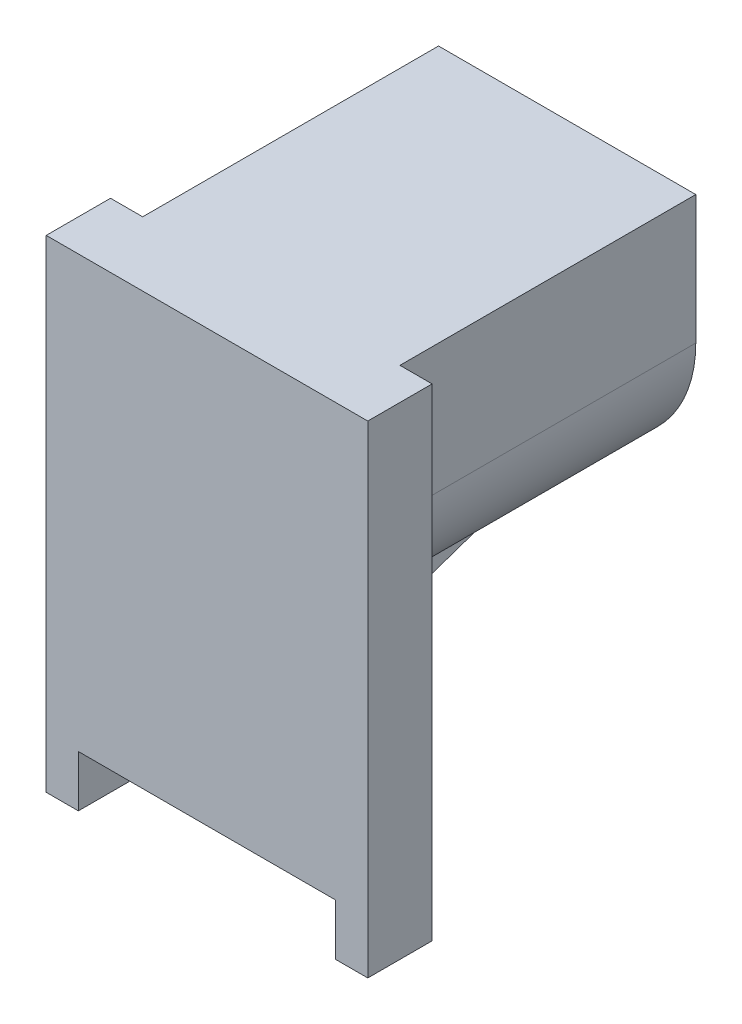
ISO-10303-21;
HEADER;
FILE_DESCRIPTION(('STEP AP214'),'2;1');
FILE_NAME('part.step','',(''),(''),'','','');
FILE_SCHEMA(('AUTOMOTIVE_DESIGN { 1 0 10303 214 1 1 1 1 }'));
ENDSEC;
DATA;
#1=APPLICATION_CONTEXT('core data for automotive mechanical design processes');
#2=APPLICATION_PROTOCOL_DEFINITION('international standard','automotive_design',2000,#1);
#3=PRODUCT_CONTEXT('',#1,'mechanical');
#4=PRODUCT('Part','Part','',(#3));
#5=PRODUCT_RELATED_PRODUCT_CATEGORY('part','',(#4));
#6=PRODUCT_DEFINITION_FORMATION('','',#4);
#7=PRODUCT_DEFINITION_CONTEXT('part definition',#1,'design');
#8=PRODUCT_DEFINITION('design','',#6,#7);
#9=PRODUCT_DEFINITION_SHAPE('','',#8);
#10=(LENGTH_UNIT() NAMED_UNIT(*) SI_UNIT(.MILLI.,.METRE.));
#11=(NAMED_UNIT(*) PLANE_ANGLE_UNIT() SI_UNIT($,.RADIAN.));
#12=(NAMED_UNIT(*) SI_UNIT($,.STERADIAN.) SOLID_ANGLE_UNIT());
#13=UNCERTAINTY_MEASURE_WITH_UNIT(LENGTH_MEASURE(1.E-05),#10,'distance_accuracy_value','');
#14=(GEOMETRIC_REPRESENTATION_CONTEXT(3) GLOBAL_UNCERTAINTY_ASSIGNED_CONTEXT((#13)) GLOBAL_UNIT_ASSIGNED_CONTEXT((#10,
#11,#12)) REPRESENTATION_CONTEXT('',''));
#15=CARTESIAN_POINT('',(0.,0.,0.));
#16=DIRECTION('',(0.,0.,1.));
#17=DIRECTION('',(1.,0.,0.));
#18=AXIS2_PLACEMENT_3D('',#15,#16,#17);
#19=CARTESIAN_POINT('',(100.,-79.3050321097279,0.));
#20=DIRECTION('',(0.,0.999971469772017,-0.00755378328999664));
#21=DIRECTION('',(0.,0.00755378328999664,0.999971469772017));
#22=AXIS2_PLACEMENT_3D('',#19,#20,#21);
#23=PLANE('',#22);
#24=DIRECTION('',(-1.,0.,0.));
#25=VECTOR('',#24,1.);
#26=CARTESIAN_POINT('',(100.,-80.,-92.));
#27=LINE('',#26,#25);
#28=CARTESIAN_POINT('',(50.,-80.,-92.));
#29=VERTEX_POINT('',#28);
#30=CARTESIAN_POINT('',(45.,-80.,-92.));
#31=VERTEX_POINT('',#30);
#32=EDGE_CURVE('E194',#29,#31,#27,.T.);
#33=ORIENTED_EDGE('',*,*,#32,.T.);
#34=DIRECTION('',(0.,-0.00755378328999664,-0.999971469772017));
#35=VECTOR('',#34,1.);
#36=CARTESIAN_POINT('',(45.,-80.,-92.));
#37=LINE('',#36,#35);
#38=CARTESIAN_POINT('',(45.,-79.6862696659689,-50.4683103566629));
#39=VERTEX_POINT('',#38);
#40=EDGE_CURVE('E69',#39,#31,#37,.T.);
#41=ORIENTED_EDGE('',*,*,#40,.F.);
#42=CARTESIAN_POINT('',(50.,-40.,5203.20867296399));
#43=DIRECTION('',(0.,0.999971469772017,-0.00755378328999664));
#44=DIRECTION('',(0.,0.00755378328999664,0.999971469772017));
#45=AXIS2_PLACEMENT_3D('',#42,#43,#44);
#46=ELLIPSE('',#45,5295.35975078493,40.);
#47=EDGE_CURVE('E190',#29,#39,#46,.T.);
#48=ORIENTED_EDGE('',*,*,#47,.F.);
#49=EDGE_LOOP('',(#33,#41,#48));
#50=FACE_BOUND('',#49,.T.);
#51=ADVANCED_FACE('F44',(#50),#23,.T.);
#52=CARTESIAN_POINT('',(100.,-80.,-92.));
#53=DIRECTION('',(0.,-0.946303433349156,-0.323279773619692));
#54=DIRECTION('',(0.,0.323279773619692,-0.946303433349156));
#55=AXIS2_PLACEMENT_3D('',#52,#53,#54);
#56=PLANE('',#55);
#57=DIRECTION('',(0.,0.323279773619692,-0.946303433349156));
#58=VECTOR('',#57,1.);
#59=CARTESIAN_POINT('',(55.,-80.,-92.));
#60=LINE('',#59,#58);
#61=CARTESIAN_POINT('',(55.,-111.429389480021,0.));
#62=VERTEX_POINT('',#61);
#63=CARTESIAN_POINT('',(55.,-80.,-92.));
#64=VERTEX_POINT('',#63);
#65=EDGE_CURVE('E58',#62,#64,#60,.T.);
#66=ORIENTED_EDGE('',*,*,#65,.F.);
#67=DIRECTION('',(-1.,0.,0.));
#68=VECTOR('',#67,1.);
#69=CARTESIAN_POINT('',(100.,-111.429389480021,0.));
#70=LINE('',#69,#68);
#71=CARTESIAN_POINT('',(45.,-111.429389480021,0.));
#72=VERTEX_POINT('',#71);
#73=EDGE_CURVE('E176',#62,#72,#70,.T.);
#74=ORIENTED_EDGE('',*,*,#73,.T.);
#75=DIRECTION('',(0.,-0.323279773619692,0.946303433349156));
#76=VECTOR('',#75,1.);
#77=CARTESIAN_POINT('',(45.,-111.429389480021,0.));
#78=LINE('',#77,#76);
#79=EDGE_CURVE('E344',#31,#72,#78,.T.);
#80=ORIENTED_EDGE('',*,*,#79,.F.);
#81=ORIENTED_EDGE('',*,*,#32,.F.);
#82=EDGE_CURVE('E185',#64,#29,#27,.T.);
#83=ORIENTED_EDGE('',*,*,#82,.F.);
#84=EDGE_LOOP('',(#66,#74,#80,#81,#83));
#85=FACE_BOUND('',#84,.T.);
#86=ADVANCED_FACE('F179',(#85),#56,.T.);
#87=CARTESIAN_POINT('',(50.,-40.,-92.));
#88=DIRECTION('',(0.,0.,1.));
#89=DIRECTION('',(1.,0.,0.));
#90=AXIS2_PLACEMENT_3D('',#87,#88,#89);
#91=CYLINDRICAL_SURFACE('',#90,40.);
#92=CARTESIAN_POINT('',(50.,-40.,0.));
#93=DIRECTION('',(0.,0.,-1.));
#94=DIRECTION('',(-1.,0.,0.));
#95=AXIS2_PLACEMENT_3D('',#92,#93,#94);
#96=CIRCLE('',#95,40.);
#97=CARTESIAN_POINT('',(90.,-40.,0.));
#98=VERTEX_POINT('',#97);
#99=CARTESIAN_POINT('',(57.4239107519726,-79.3050321097279,0.));
#100=VERTEX_POINT('',#99);
#101=EDGE_CURVE('E220',#98,#100,#96,.T.);
#102=ORIENTED_EDGE('',*,*,#101,.T.);
#103=CARTESIAN_POINT('',(55.,-79.6862696659689,-50.4683103566629));
#104=VERTEX_POINT('',#103);
#105=EDGE_CURVE('E195',#100,#104,#46,.T.);
#106=ORIENTED_EDGE('',*,*,#105,.T.);
#107=EDGE_CURVE('E186',#104,#29,#46,.T.);
#108=ORIENTED_EDGE('',*,*,#107,.T.);
#109=CARTESIAN_POINT('',(50.,-40.,-92.));
#110=DIRECTION('',(0.,0.,-1.));
#111=DIRECTION('',(-1.,0.,0.));
#112=AXIS2_PLACEMENT_3D('',#109,#110,#111);
#113=CIRCLE('',#112,40.);
#114=CARTESIAN_POINT('',(90.,-40.,-92.));
#115=VERTEX_POINT('',#114);
#116=EDGE_CURVE('E206',#115,#29,#113,.T.);
#117=ORIENTED_EDGE('',*,*,#116,.F.);
#118=DIRECTION('',(0.,0.,1.));
#119=VECTOR('',#118,1.);
#120=CARTESIAN_POINT('',(90.,-40.,-92.));
#121=LINE('',#120,#119);
#122=EDGE_CURVE('E216',#115,#98,#121,.T.);
#123=ORIENTED_EDGE('',*,*,#122,.T.);
#124=EDGE_LOOP('',(#102,#106,#108,#117,#123));
#125=FACE_BOUND('',#124,.T.);
#126=ADVANCED_FACE('F358',(#125),#91,.T.);
#127=CARTESIAN_POINT('',(0.,-150.,20.));
#128=DIRECTION('',(1.,0.,0.));
#129=DIRECTION('',(0.,0.,-1.));
#130=AXIS2_PLACEMENT_3D('',#127,#128,#129);
#131=PLANE('',#130);
#132=DIRECTION('',(0.,-1.,0.));
#133=VECTOR('',#132,1.);
#134=CARTESIAN_POINT('',(0.,-150.,0.));
#135=LINE('',#134,#133);
#136=CARTESIAN_POINT('',(0.,0.,0.));
#137=VERTEX_POINT('',#136);
#138=CARTESIAN_POINT('',(0.,-150.,0.));
#139=VERTEX_POINT('',#138);
#140=EDGE_CURVE('E240',#137,#139,#135,.T.);
#141=ORIENTED_EDGE('',*,*,#140,.T.);
#142=DIRECTION('',(0.,0.,-1.));
#143=VECTOR('',#142,1.);
#144=CARTESIAN_POINT('',(0.,-150.,20.));
#145=LINE('',#144,#143);
#146=CARTESIAN_POINT('',(0.,-150.,20.));
#147=VERTEX_POINT('',#146);
#148=EDGE_CURVE('E11',#147,#139,#145,.T.);
#149=ORIENTED_EDGE('',*,*,#148,.F.);
#150=DIRECTION('',(0.,-1.,0.));
#151=VECTOR('',#150,1.);
#152=CARTESIAN_POINT('',(0.,-150.,20.));
#153=LINE('',#152,#151);
#154=CARTESIAN_POINT('',(0.,0.,20.));
#155=VERTEX_POINT('',#154);
#156=EDGE_CURVE('E236',#155,#147,#153,.T.);
#157=ORIENTED_EDGE('',*,*,#156,.F.);
#158=DIRECTION('',(0.,0.,-1.));
#159=VECTOR('',#158,1.);
#160=CARTESIAN_POINT('',(0.,0.,20.));
#161=LINE('',#160,#159);
#162=EDGE_CURVE('E258',#155,#137,#161,.T.);
#163=ORIENTED_EDGE('',*,*,#162,.T.);
#164=EDGE_LOOP('',(#141,#149,#157,#163));
#165=FACE_BOUND('',#164,.T.);
#166=ADVANCED_FACE('F50',(#165),#131,.F.);
#167=CARTESIAN_POINT('',(10.,-150.,20.));
#168=DIRECTION('',(0.,1.,0.));
#169=DIRECTION('',(0.,0.,1.));
#170=AXIS2_PLACEMENT_3D('',#167,#168,#169);
#171=PLANE('',#170);
#172=DIRECTION('',(1.,0.,0.));
#173=VECTOR('',#172,1.);
#174=CARTESIAN_POINT('',(10.,-150.,0.));
#175=LINE('',#174,#173);
#176=CARTESIAN_POINT('',(10.,-150.,0.));
#177=VERTEX_POINT('',#176);
#178=EDGE_CURVE('E256',#139,#177,#175,.T.);
#179=ORIENTED_EDGE('',*,*,#178,.T.);
#180=DIRECTION('',(0.,0.,-1.));
#181=VECTOR('',#180,1.);
#182=CARTESIAN_POINT('',(10.,-150.,20.));
#183=LINE('',#182,#181);
#184=CARTESIAN_POINT('',(10.,-150.,20.));
#185=VERTEX_POINT('',#184);
#186=EDGE_CURVE('E52',#185,#177,#183,.T.);
#187=ORIENTED_EDGE('',*,*,#186,.F.);
#188=DIRECTION('',(1.,0.,0.));
#189=VECTOR('',#188,1.);
#190=CARTESIAN_POINT('',(10.,-150.,20.));
#191=LINE('',#190,#189);
#192=EDGE_CURVE('E242',#147,#185,#191,.T.);
#193=ORIENTED_EDGE('',*,*,#192,.F.);
#194=ORIENTED_EDGE('',*,*,#148,.T.);
#195=EDGE_LOOP('',(#179,#187,#193,#194));
#196=FACE_BOUND('',#195,.T.);
#197=ADVANCED_FACE('F316',(#196),#171,.F.);
#198=CARTESIAN_POINT('',(10.,-134.,20.));
#199=DIRECTION('',(-1.,0.,0.));
#200=DIRECTION('',(0.,0.,1.));
#201=AXIS2_PLACEMENT_3D('',#198,#199,#200);
#202=PLANE('',#201);
#203=DIRECTION('',(0.,1.,0.));
#204=VECTOR('',#203,1.);
#205=CARTESIAN_POINT('',(10.,-134.,0.));
#206=LINE('',#205,#204);
#207=CARTESIAN_POINT('',(10.,-134.,0.));
#208=VERTEX_POINT('',#207);
#209=EDGE_CURVE('E257',#177,#208,#206,.T.);
#210=ORIENTED_EDGE('',*,*,#209,.T.);
#211=DIRECTION('',(0.,0.,-1.));
#212=VECTOR('',#211,1.);
#213=CARTESIAN_POINT('',(10.,-134.,20.));
#214=LINE('',#213,#212);
#215=CARTESIAN_POINT('',(10.,-134.,20.));
#216=VERTEX_POINT('',#215);
#217=EDGE_CURVE('E290',#216,#208,#214,.T.);
#218=ORIENTED_EDGE('',*,*,#217,.F.);
#219=DIRECTION('',(0.,1.,0.));
#220=VECTOR('',#219,1.);
#221=CARTESIAN_POINT('',(10.,-134.,20.));
#222=LINE('',#221,#220);
#223=EDGE_CURVE('E244',#185,#216,#222,.T.);
#224=ORIENTED_EDGE('',*,*,#223,.F.);
#225=ORIENTED_EDGE('',*,*,#186,.T.);
#226=EDGE_LOOP('',(#210,#218,#224,#225));
#227=FACE_BOUND('',#226,.T.);
#228=ADVANCED_FACE('F294',(#227),#202,.F.);
#229=CARTESIAN_POINT('',(90.,-134.,20.));
#230=DIRECTION('',(0.,1.,0.));
#231=DIRECTION('',(0.,0.,1.));
#232=AXIS2_PLACEMENT_3D('',#229,#230,#231);
#233=PLANE('',#232);
#234=DIRECTION('',(1.,0.,0.));
#235=VECTOR('',#234,1.);
#236=CARTESIAN_POINT('',(90.,-134.,0.));
#237=LINE('',#236,#235);
#238=CARTESIAN_POINT('',(90.,-134.,0.));
#239=VERTEX_POINT('',#238);
#240=EDGE_CURVE('E265',#208,#239,#237,.T.);
#241=ORIENTED_EDGE('',*,*,#240,.T.);
#242=DIRECTION('',(0.,0.,-1.));
#243=VECTOR('',#242,1.);
#244=CARTESIAN_POINT('',(90.,-134.,20.));
#245=LINE('',#244,#243);
#246=CARTESIAN_POINT('',(90.,-134.,20.));
#247=VERTEX_POINT('',#246);
#248=EDGE_CURVE('E284',#247,#239,#245,.T.);
#249=ORIENTED_EDGE('',*,*,#248,.F.);
#250=DIRECTION('',(1.,0.,0.));
#251=VECTOR('',#250,1.);
#252=CARTESIAN_POINT('',(90.,-134.,20.));
#253=LINE('',#252,#251);
#254=EDGE_CURVE('E247',#216,#247,#253,.T.);
#255=ORIENTED_EDGE('',*,*,#254,.F.);
#256=ORIENTED_EDGE('',*,*,#217,.T.);
#257=EDGE_LOOP('',(#241,#249,#255,#256));
#258=FACE_BOUND('',#257,.T.);
#259=ADVANCED_FACE('F301',(#258),#233,.F.);
#260=CARTESIAN_POINT('',(90.,-150.,20.));
#261=DIRECTION('',(1.,0.,0.));
#262=DIRECTION('',(0.,0.,-1.));
#263=AXIS2_PLACEMENT_3D('',#260,#261,#262);
#264=PLANE('',#263);
#265=DIRECTION('',(0.,-1.,0.));
#266=VECTOR('',#265,1.);
#267=CARTESIAN_POINT('',(90.,-150.,0.));
#268=LINE('',#267,#266);
#269=CARTESIAN_POINT('',(90.,-150.,0.));
#270=VERTEX_POINT('',#269);
#271=EDGE_CURVE('E262',#239,#270,#268,.T.);
#272=ORIENTED_EDGE('',*,*,#271,.T.);
#273=DIRECTION('',(0.,0.,-1.));
#274=VECTOR('',#273,1.);
#275=CARTESIAN_POINT('',(90.,-150.,20.));
#276=LINE('',#275,#274);
#277=CARTESIAN_POINT('',(90.,-150.,20.));
#278=VERTEX_POINT('',#277);
#279=EDGE_CURVE('E282',#278,#270,#276,.T.);
#280=ORIENTED_EDGE('',*,*,#279,.F.);
#281=DIRECTION('',(0.,-1.,0.));
#282=VECTOR('',#281,1.);
#283=CARTESIAN_POINT('',(90.,-150.,20.));
#284=LINE('',#283,#282);
#285=EDGE_CURVE('E249',#247,#278,#284,.T.);
#286=ORIENTED_EDGE('',*,*,#285,.F.);
#287=ORIENTED_EDGE('',*,*,#248,.T.);
#288=EDGE_LOOP('',(#272,#280,#286,#287));
#289=FACE_BOUND('',#288,.T.);
#290=ADVANCED_FACE('F306',(#289),#264,.F.);
#291=CARTESIAN_POINT('',(100.,-150.,20.));
#292=DIRECTION('',(0.,1.,0.));
#293=DIRECTION('',(0.,0.,1.));
#294=AXIS2_PLACEMENT_3D('',#291,#292,#293);
#295=PLANE('',#294);
#296=DIRECTION('',(1.,0.,0.));
#297=VECTOR('',#296,1.);
#298=CARTESIAN_POINT('',(100.,-150.,0.));
#299=LINE('',#298,#297);
#300=CARTESIAN_POINT('',(100.,-150.,0.));
#301=VERTEX_POINT('',#300);
#302=EDGE_CURVE('E266',#270,#301,#299,.T.);
#303=ORIENTED_EDGE('',*,*,#302,.T.);
#304=DIRECTION('',(0.,0.,-1.));
#305=VECTOR('',#304,1.);
#306=CARTESIAN_POINT('',(100.,-150.,20.));
#307=LINE('',#306,#305);
#308=CARTESIAN_POINT('',(100.,-150.,20.));
#309=VERTEX_POINT('',#308);
#310=EDGE_CURVE('E279',#309,#301,#307,.T.);
#311=ORIENTED_EDGE('',*,*,#310,.F.);
#312=DIRECTION('',(1.,0.,0.));
#313=VECTOR('',#312,1.);
#314=CARTESIAN_POINT('',(100.,-150.,20.));
#315=LINE('',#314,#313);
#316=EDGE_CURVE('E248',#278,#309,#315,.T.);
#317=ORIENTED_EDGE('',*,*,#316,.F.);
#318=ORIENTED_EDGE('',*,*,#279,.T.);
#319=EDGE_LOOP('',(#303,#311,#317,#318));
#320=FACE_BOUND('',#319,.T.);
#321=ADVANCED_FACE('F429',(#320),#295,.F.);
#322=CARTESIAN_POINT('',(100.,0.,20.));
#323=DIRECTION('',(-1.,0.,0.));
#324=DIRECTION('',(0.,0.,1.));
#325=AXIS2_PLACEMENT_3D('',#322,#323,#324);
#326=PLANE('',#325);
#327=DIRECTION('',(0.,1.,0.));
#328=VECTOR('',#327,1.);
#329=CARTESIAN_POINT('',(100.,0.,0.));
#330=LINE('',#329,#328);
#331=CARTESIAN_POINT('',(100.,0.,0.));
#332=VERTEX_POINT('',#331);
#333=EDGE_CURVE('E268',#301,#332,#330,.T.);
#334=ORIENTED_EDGE('',*,*,#333,.T.);
#335=DIRECTION('',(0.,0.,-1.));
#336=VECTOR('',#335,1.);
#337=CARTESIAN_POINT('',(100.,0.,20.));
#338=LINE('',#337,#336);
#339=CARTESIAN_POINT('',(100.,0.,20.));
#340=VERTEX_POINT('',#339);
#341=EDGE_CURVE('E274',#340,#332,#338,.T.);
#342=ORIENTED_EDGE('',*,*,#341,.F.);
#343=DIRECTION('',(0.,1.,0.));
#344=VECTOR('',#343,1.);
#345=CARTESIAN_POINT('',(100.,0.,20.));
#346=LINE('',#345,#344);
#347=EDGE_CURVE('E252',#309,#340,#346,.T.);
#348=ORIENTED_EDGE('',*,*,#347,.F.);
#349=ORIENTED_EDGE('',*,*,#310,.T.);
#350=EDGE_LOOP('',(#334,#342,#348,#349));
#351=FACE_BOUND('',#350,.T.);
#352=ADVANCED_FACE('F426',(#351),#326,.F.);
#353=CARTESIAN_POINT('',(0.,0.,20.));
#354=DIRECTION('',(0.,-1.,0.));
#355=DIRECTION('',(0.,0.,-1.));
#356=AXIS2_PLACEMENT_3D('',#353,#354,#355);
#357=PLANE('',#356);
#358=DIRECTION('',(-1.,0.,0.));
#359=VECTOR('',#358,1.);
#360=CARTESIAN_POINT('',(0.,0.,0.));
#361=LINE('',#360,#359);
#362=CARTESIAN_POINT('',(90.,0.,0.));
#363=VERTEX_POINT('',#362);
#364=EDGE_CURVE('E245',#332,#363,#361,.T.);
#365=ORIENTED_EDGE('',*,*,#364,.T.);
#366=DIRECTION('',(0.,0.,1.));
#367=VECTOR('',#366,1.);
#368=CARTESIAN_POINT('',(90.,0.,-92.));
#369=LINE('',#368,#367);
#370=CARTESIAN_POINT('',(90.,0.,-92.));
#371=VERTEX_POINT('',#370);
#372=EDGE_CURVE('E228',#371,#363,#369,.T.);
#373=ORIENTED_EDGE('',*,*,#372,.F.);
#374=DIRECTION('',(1.,0.,0.));
#375=VECTOR('',#374,1.);
#376=CARTESIAN_POINT('',(10.,0.,-92.));
#377=LINE('',#376,#375);
#378=CARTESIAN_POINT('',(10.,0.,-92.));
#379=VERTEX_POINT('',#378);
#380=EDGE_CURVE('E215',#379,#371,#377,.T.);
#381=ORIENTED_EDGE('',*,*,#380,.F.);
#382=DIRECTION('',(0.,0.,1.));
#383=VECTOR('',#382,1.);
#384=CARTESIAN_POINT('',(10.,0.,-92.));
#385=LINE('',#384,#383);
#386=CARTESIAN_POINT('',(10.,0.,0.));
#387=VERTEX_POINT('',#386);
#388=EDGE_CURVE('E232',#379,#387,#385,.T.);
#389=ORIENTED_EDGE('',*,*,#388,.T.);
#390=EDGE_CURVE('E269',#387,#137,#361,.T.);
#391=ORIENTED_EDGE('',*,*,#390,.T.);
#392=ORIENTED_EDGE('',*,*,#162,.F.);
#393=DIRECTION('',(-1.,0.,0.));
#394=VECTOR('',#393,1.);
#395=CARTESIAN_POINT('',(0.,0.,20.));
#396=LINE('',#395,#394);
#397=EDGE_CURVE('E255',#340,#155,#396,.T.);
#398=ORIENTED_EDGE('',*,*,#397,.F.);
#399=ORIENTED_EDGE('',*,*,#341,.T.);
#400=EDGE_LOOP('',(#365,#373,#381,#389,#391,#392,#398,#399));
#401=FACE_BOUND('',#400,.T.);
#402=ADVANCED_FACE('F327',(#401),#357,.F.);
#403=CARTESIAN_POINT('',(0.,0.,20.));
#404=DIRECTION('',(0.,0.,-1.));
#405=DIRECTION('',(-1.,0.,0.));
#406=AXIS2_PLACEMENT_3D('',#403,#404,#405);
#407=PLANE('',#406);
#408=ORIENTED_EDGE('',*,*,#156,.T.);
#409=ORIENTED_EDGE('',*,*,#192,.T.);
#410=ORIENTED_EDGE('',*,*,#223,.T.);
#411=ORIENTED_EDGE('',*,*,#254,.T.);
#412=ORIENTED_EDGE('',*,*,#285,.T.);
#413=ORIENTED_EDGE('',*,*,#316,.T.);
#414=ORIENTED_EDGE('',*,*,#347,.T.);
#415=ORIENTED_EDGE('',*,*,#397,.T.);
#416=EDGE_LOOP('',(#408,#409,#410,#411,#412,#413,#414,#415));
#417=FACE_BOUND('',#416,.T.);
#418=ADVANCED_FACE('F315',(#417),#407,.F.);
#419=CARTESIAN_POINT('',(0.,0.,0.));
#420=DIRECTION('',(0.,0.,-1.));
#421=DIRECTION('',(-1.,0.,0.));
#422=AXIS2_PLACEMENT_3D('',#419,#420,#421);
#423=PLANE('',#422);
#424=ORIENTED_EDGE('',*,*,#73,.F.);
#425=DIRECTION('',(0.,-1.,0.));
#426=VECTOR('',#425,1.);
#427=CARTESIAN_POINT('',(55.,-111.429389480021,0.));
#428=LINE('',#427,#426);
#429=CARTESIAN_POINT('',(55.,-79.3050321097279,0.));
#430=VERTEX_POINT('',#429);
#431=EDGE_CURVE('E169',#430,#62,#428,.T.);
#432=ORIENTED_EDGE('',*,*,#431,.F.);
#433=DIRECTION('',(1.,0.,0.));
#434=VECTOR('',#433,1.);
#435=CARTESIAN_POINT('',(55.,-79.3050321097279,0.));
#436=LINE('',#435,#434);
#437=EDGE_CURVE('E349',#430,#100,#436,.T.);
#438=ORIENTED_EDGE('',*,*,#437,.T.);
#439=ORIENTED_EDGE('',*,*,#101,.F.);
#440=DIRECTION('',(0.,-1.,0.));
#441=VECTOR('',#440,1.);
#442=CARTESIAN_POINT('',(90.,0.,0.));
#443=LINE('',#442,#441);
#444=EDGE_CURVE('E224',#363,#98,#443,.T.);
#445=ORIENTED_EDGE('',*,*,#444,.F.);
#446=ORIENTED_EDGE('',*,*,#364,.F.);
#447=ORIENTED_EDGE('',*,*,#333,.F.);
#448=ORIENTED_EDGE('',*,*,#302,.F.);
#449=ORIENTED_EDGE('',*,*,#271,.F.);
#450=ORIENTED_EDGE('',*,*,#240,.F.);
#451=ORIENTED_EDGE('',*,*,#209,.F.);
#452=ORIENTED_EDGE('',*,*,#178,.F.);
#453=ORIENTED_EDGE('',*,*,#140,.F.);
#454=ORIENTED_EDGE('',*,*,#390,.F.);
#455=DIRECTION('',(0.,1.,0.));
#456=VECTOR('',#455,1.);
#457=CARTESIAN_POINT('',(10.,-40.,0.));
#458=LINE('',#457,#456);
#459=CARTESIAN_POINT('',(10.,-40.,0.));
#460=VERTEX_POINT('',#459);
#461=EDGE_CURVE('E219',#460,#387,#458,.T.);
#462=ORIENTED_EDGE('',*,*,#461,.F.);
#463=CARTESIAN_POINT('',(42.5760892480275,-79.3050321097279,0.));
#464=VERTEX_POINT('',#463);
#465=EDGE_CURVE('E205',#464,#460,#96,.T.);
#466=ORIENTED_EDGE('',*,*,#465,.F.);
#467=DIRECTION('',(-1.,0.,0.));
#468=VECTOR('',#467,1.);
#469=CARTESIAN_POINT('',(45.,-79.3050321097279,0.));
#470=LINE('',#469,#468);
#471=CARTESIAN_POINT('',(45.,-79.3050321097279,0.));
#472=VERTEX_POINT('',#471);
#473=EDGE_CURVE('E338',#472,#464,#470,.T.);
#474=ORIENTED_EDGE('',*,*,#473,.F.);
#475=DIRECTION('',(0.,1.,0.));
#476=VECTOR('',#475,1.);
#477=CARTESIAN_POINT('',(45.,-79.3050321097279,0.));
#478=LINE('',#477,#476);
#479=EDGE_CURVE('E187',#72,#472,#478,.T.);
#480=ORIENTED_EDGE('',*,*,#479,.F.);
#481=EDGE_LOOP('',(#424,#432,#438,#439,#445,#446,#447,#448,#449,#450,#451,#452,#453,#454,#462,
#466,#474,#480));
#482=FACE_BOUND('',#481,.T.);
#483=ADVANCED_FACE('F184',(#482),#423,.T.);
#484=CARTESIAN_POINT('',(10.,-40.,-92.));
#485=VERTEX_POINT('',#484);
#486=EDGE_CURVE('E209',#29,#485,#113,.T.);
#487=ORIENTED_EDGE('',*,*,#486,.F.);
#488=ORIENTED_EDGE('',*,*,#47,.T.);
#489=CARTESIAN_POINT('',(50.,-40.,5203.20867296399));
#490=DIRECTION('',(0.,0.999971469772017,-0.00755378328999664));
#491=DIRECTION('',(0.,0.00755378328999664,0.999971469772017));
#492=AXIS2_PLACEMENT_3D('',#489,#490,#491);
#493=ELLIPSE('',#492,5295.35975078493,40.);
#494=EDGE_CURVE('E198',#39,#464,#493,.T.);
#495=ORIENTED_EDGE('',*,*,#494,.T.);
#496=ORIENTED_EDGE('',*,*,#465,.T.);
#497=DIRECTION('',(0.,0.,1.));
#498=VECTOR('',#497,1.);
#499=CARTESIAN_POINT('',(10.,-40.,-92.));
#500=LINE('',#499,#498);
#501=EDGE_CURVE('E231',#485,#460,#500,.T.);
#502=ORIENTED_EDGE('',*,*,#501,.F.);
#503=EDGE_LOOP('',(#487,#488,#495,#496,#502));
#504=FACE_BOUND('',#503,.T.);
#505=ADVANCED_FACE('F337',(#504),#91,.T.);
#506=CARTESIAN_POINT('',(10.,-40.,-92.));
#507=DIRECTION('',(1.,0.,0.));
#508=DIRECTION('',(0.,1.,0.));
#509=AXIS2_PLACEMENT_3D('',#506,#507,#508);
#510=PLANE('',#509);
#511=ORIENTED_EDGE('',*,*,#461,.T.);
#512=ORIENTED_EDGE('',*,*,#388,.F.);
#513=DIRECTION('',(0.,1.,0.));
#514=VECTOR('',#513,1.);
#515=CARTESIAN_POINT('',(10.,-40.,-92.));
#516=LINE('',#515,#514);
#517=EDGE_CURVE('E207',#485,#379,#516,.T.);
#518=ORIENTED_EDGE('',*,*,#517,.F.);
#519=ORIENTED_EDGE('',*,*,#501,.T.);
#520=EDGE_LOOP('',(#511,#512,#518,#519));
#521=FACE_BOUND('',#520,.T.);
#522=ADVANCED_FACE('F322',(#521),#510,.F.);
#523=CARTESIAN_POINT('',(90.,0.,-92.));
#524=DIRECTION('',(-1.,0.,0.));
#525=DIRECTION('',(0.,0.,1.));
#526=AXIS2_PLACEMENT_3D('',#523,#524,#525);
#527=PLANE('',#526);
#528=ORIENTED_EDGE('',*,*,#444,.T.);
#529=ORIENTED_EDGE('',*,*,#122,.F.);
#530=DIRECTION('',(0.,-1.,0.));
#531=VECTOR('',#530,1.);
#532=CARTESIAN_POINT('',(90.,0.,-92.));
#533=LINE('',#532,#531);
#534=EDGE_CURVE('E212',#371,#115,#533,.T.);
#535=ORIENTED_EDGE('',*,*,#534,.F.);
#536=ORIENTED_EDGE('',*,*,#372,.T.);
#537=EDGE_LOOP('',(#528,#529,#535,#536));
#538=FACE_BOUND('',#537,.T.);
#539=ADVANCED_FACE('F364',(#538),#527,.F.);
#540=CARTESIAN_POINT('',(50.,-40.,-92.));
#541=DIRECTION('',(0.,0.,-1.));
#542=DIRECTION('',(-1.,0.,0.));
#543=AXIS2_PLACEMENT_3D('',#540,#541,#542);
#544=PLANE('',#543);
#545=CARTESIAN_POINT('',(50.,-40.,-92.));
#546=DIRECTION('',(0.,0.,-1.));
#547=DIRECTION('',(-1.,0.,0.));
#548=AXIS2_PLACEMENT_3D('',#545,#546,#547);
#549=CIRCLE('',#548,24.);
#550=CARTESIAN_POINT('',(26.,-40.,-92.));
#551=VERTEX_POINT('',#550);
#552=EDGE_CURVE('E201',#551,#551,#549,.T.);
#553=ORIENTED_EDGE('',*,*,#552,.F.);
#554=EDGE_LOOP('',(#553));
#555=FACE_BOUND('',#554,.T.);
#556=ORIENTED_EDGE('',*,*,#116,.T.);
#557=ORIENTED_EDGE('',*,*,#486,.T.);
#558=ORIENTED_EDGE('',*,*,#517,.T.);
#559=ORIENTED_EDGE('',*,*,#380,.T.);
#560=ORIENTED_EDGE('',*,*,#534,.T.);
#561=EDGE_LOOP('',(#556,#557,#558,#559,#560));
#562=FACE_BOUND('',#561,.T.);
#563=ADVANCED_FACE('F335',(#555,#562),#544,.T.);
#564=CARTESIAN_POINT('',(50.,-40.,0.));
#565=DIRECTION('',(0.,0.,-1.));
#566=DIRECTION('',(-1.,0.,0.));
#567=AXIS2_PLACEMENT_3D('',#564,#565,#566);
#568=CYLINDRICAL_SURFACE('',#567,24.);
#569=CARTESIAN_POINT('',(50.,-40.,0.));
#570=DIRECTION('',(0.,0.,-1.));
#571=DIRECTION('',(-1.,0.,0.));
#572=AXIS2_PLACEMENT_3D('',#569,#570,#571);
#573=CIRCLE('',#572,24.);
#574=CARTESIAN_POINT('',(26.,-40.,0.));
#575=VERTEX_POINT('',#574);
#576=EDGE_CURVE('E200',#575,#575,#573,.T.);
#577=ORIENTED_EDGE('',*,*,#576,.F.);
#578=EDGE_LOOP('',(#577));
#579=FACE_BOUND('',#578,.T.);
#580=ORIENTED_EDGE('',*,*,#552,.T.);
#581=EDGE_LOOP('',(#580));
#582=FACE_BOUND('',#581,.T.);
#583=ADVANCED_FACE('F375',(#579,#582),#568,.F.);
#584=CARTESIAN_POINT('',(50.,-40.,0.));
#585=DIRECTION('',(0.,0.,-1.));
#586=DIRECTION('',(-1.,0.,0.));
#587=AXIS2_PLACEMENT_3D('',#584,#585,#586);
#588=PLANE('',#587);
#589=ORIENTED_EDGE('',*,*,#576,.T.);
#590=EDGE_LOOP('',(#589));
#591=FACE_BOUND('',#590,.T.);
#592=ADVANCED_FACE('F387',(#591),#588,.T.);
#593=DIRECTION('',(0.,0.00755378328999664,0.999971469772017));
#594=VECTOR('',#593,1.);
#595=CARTESIAN_POINT('',(55.,-79.3050321097279,0.));
#596=LINE('',#595,#594);
#597=EDGE_CURVE('E352',#64,#104,#596,.T.);
#598=ORIENTED_EDGE('',*,*,#597,.F.);
#599=ORIENTED_EDGE('',*,*,#82,.T.);
#600=ORIENTED_EDGE('',*,*,#107,.F.);
#601=EDGE_LOOP('',(#598,#599,#600));
#602=FACE_BOUND('',#601,.T.);
#603=ADVANCED_FACE('F357',(#602),#23,.T.);
#604=CARTESIAN_POINT('',(45.,-80.,-92.));
#605=DIRECTION('',(0.,0.999971469772017,-0.00755378328999664));
#606=DIRECTION('',(0.,0.00755378328999664,0.999971469772017));
#607=AXIS2_PLACEMENT_3D('',#604,#605,#606);
#608=PLANE('',#607);
#609=EDGE_CURVE('E342',#472,#39,#37,.T.);
#610=ORIENTED_EDGE('',*,*,#609,.F.);
#611=ORIENTED_EDGE('',*,*,#473,.T.);
#612=ORIENTED_EDGE('',*,*,#494,.F.);
#613=EDGE_LOOP('',(#610,#611,#612));
#614=FACE_BOUND('',#613,.T.);
#615=ADVANCED_FACE('F343',(#614),#608,.F.);
#616=CARTESIAN_POINT('',(45.,0.,0.));
#617=DIRECTION('',(-1.,0.,0.));
#618=DIRECTION('',(0.,0.,1.));
#619=AXIS2_PLACEMENT_3D('',#616,#617,#618);
#620=PLANE('',#619);
#621=ORIENTED_EDGE('',*,*,#79,.T.);
#622=ORIENTED_EDGE('',*,*,#479,.T.);
#623=ORIENTED_EDGE('',*,*,#609,.T.);
#624=ORIENTED_EDGE('',*,*,#40,.T.);
#625=EDGE_LOOP('',(#621,#622,#623,#624));
#626=FACE_BOUND('',#625,.T.);
#627=ADVANCED_FACE('F345',(#626),#620,.T.);
#628=CARTESIAN_POINT('',(55.,-79.3050321097279,0.));
#629=DIRECTION('',(0.,0.999971469772017,-0.00755378328999664));
#630=DIRECTION('',(0.,0.00755378328999664,0.999971469772017));
#631=AXIS2_PLACEMENT_3D('',#628,#629,#630);
#632=PLANE('',#631);
#633=ORIENTED_EDGE('',*,*,#437,.F.);
#634=EDGE_CURVE('E168',#104,#430,#596,.T.);
#635=ORIENTED_EDGE('',*,*,#634,.F.);
#636=ORIENTED_EDGE('',*,*,#105,.F.);
#637=EDGE_LOOP('',(#633,#635,#636));
#638=FACE_BOUND('',#637,.T.);
#639=ADVANCED_FACE('F362',(#638),#632,.F.);
#640=CARTESIAN_POINT('',(55.,0.,0.));
#641=DIRECTION('',(-1.,0.,0.));
#642=DIRECTION('',(0.,0.,1.));
#643=AXIS2_PLACEMENT_3D('',#640,#641,#642);
#644=PLANE('',#643);
#645=ORIENTED_EDGE('',*,*,#431,.T.);
#646=ORIENTED_EDGE('',*,*,#65,.T.);
#647=ORIENTED_EDGE('',*,*,#597,.T.);
#648=ORIENTED_EDGE('',*,*,#634,.T.);
#649=EDGE_LOOP('',(#645,#646,#647,#648));
#650=FACE_BOUND('',#649,.T.);
#651=ADVANCED_FACE('F166',(#650),#644,.F.);
#652=CLOSED_SHELL('',(#51,#86,#126,#166,#197,#228,#259,#290,#321,#352,#402,#418,#483,#505,#522,
#539,#563,#583,#592,#603,#615,#627,#639,#651));
#653=MANIFOLD_SOLID_BREP('B2',#652);
#654=ADVANCED_BREP_SHAPE_REPRESENTATION('',(#18,#653),#14);
#655=SHAPE_DEFINITION_REPRESENTATION(#9,#654);
ENDSEC;
END-ISO-10303-21;
